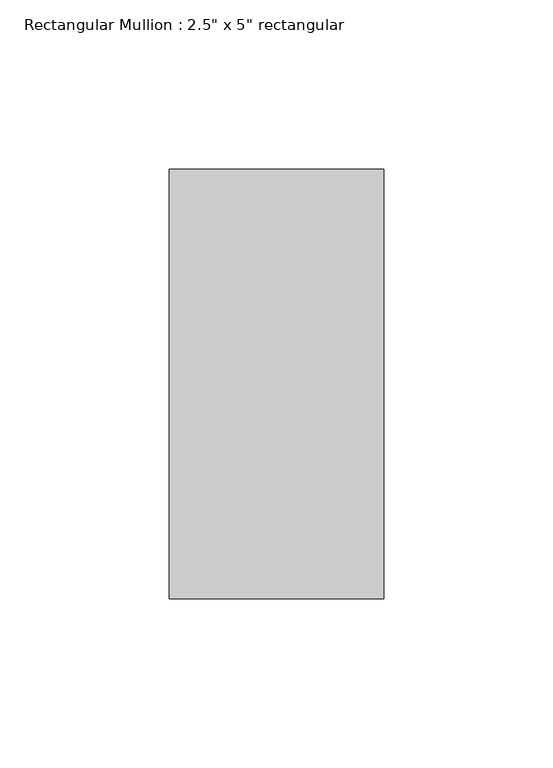
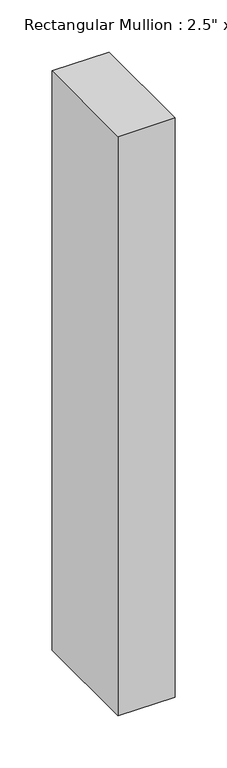
"""IFC4 building model written with IfcOpenShell, lengths in millimetres: member geometry."""

from ifc_helpers import new_model, si_unit, frame, origin, place, context, project, spatial, polyline, outline, extrude, source, transform, mapped, element, save


def member_d6240b74(model_context):
    return source(origin(), model_context, "Body", "SweptSolid", [
        extrude(outline(polyline([(31.75, 63.5), (31.75, -63.5), (-31.75, -63.5), (-31.75, 63.5), (31.75, 63.5)])), frame((0.0, 0.0, -680.0388769), z_axis=(0.0, 0.0, 1.0), x_axis=(1.0, 0.0, 0.0)), (0.0, 0.0, 1.0), 680.0388769),
    ])


if __name__ == "__main__":
    model = new_model("IFC4")
    model_context = context("Model", 3, world=origin())
    ifc_project = project(units=[si_unit("LENGTHUNIT", "METRE", prefix="MILLI")], contexts=[model_context])
    site = spatial("IfcSite", under=ifc_project)
    building = spatial("IfcBuilding", under=site)
    placement = place(None, origin())
    member_shape = member_d6240b74(model_context)
    element("IfcMember", 1, ObjectType="Rectangular Mullion : 2.5\" x 5\" rectangular", at=placement, inside=building, context=model_context, shape_type="MappedRepresentation", body=[
        mapped(member_shape, transform((0.0, 0.0, 0.0), x_axis=(1.0, 0.0, 0.0), y_axis=(0.0, 1.0, 0.0), z_axis=(0.0, 0.0, 1.0))),
    ])
    save(model, "model.ifc")

# Revit data of these elements
# Type "Rectangular Mullion : 2.5\" x 5\" rectangular"
#   built-in parameter 1007304 = 0.416667 (stored number, unit not read)
#   built-in parameter 1007301 = 0.104167 (stored number, unit not read)
#   built-in parameter 1007300 = 0.104167 (stored number, unit not read)
# Element 1 (IfcMember, "Rectangular Mullion : 2.5\" x 5\" rectangular")
#   Materials on its faces: "Aluminum"
# Materials
#   "Aluminum": class "Metal", colour RGB 247 247 247, transparency 0, Description = "Aluminum 6061", Cost = 0
